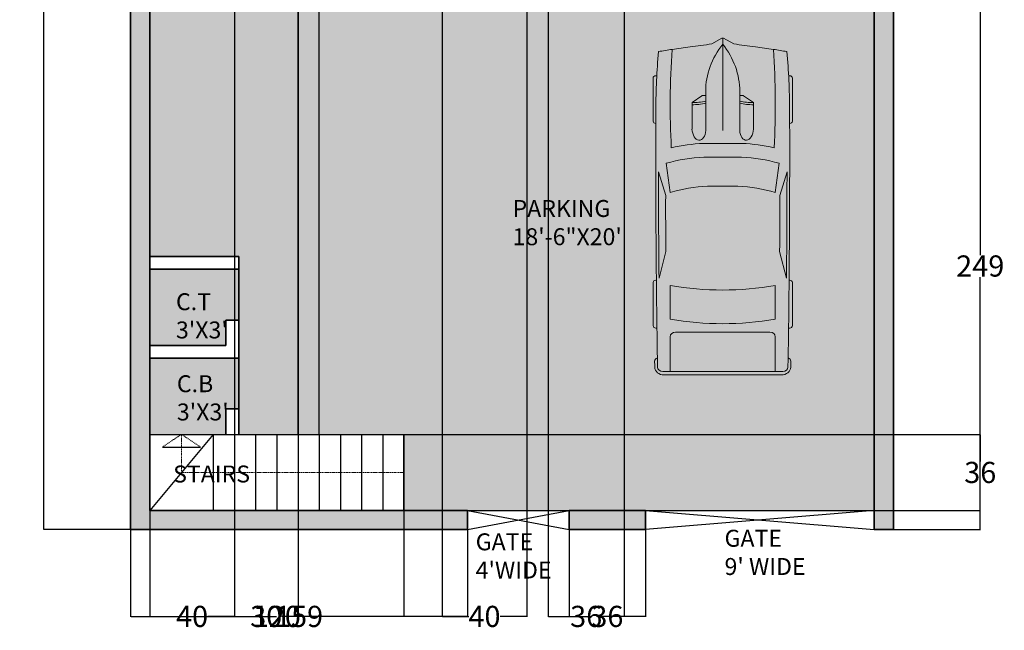
# Model space of a CAD drawing. Units: inches. Extents: x 286 to 756, y 360 to 1175.
# Tile 1 of 4: x 286 to 750, y 360 to 649. Entities that reach past the tile are written whole.
import ezdxf

# ---------------------------------------------------------------- set-up
doc = ezdxf.new("R2010")
doc.units = ezdxf.units.IN
doc.header["$MEASUREMENT"] = 0
doc.linetypes.add('DASHED', pattern=[0.75, 0.5, -0.25])
for name, color, linetype, lineweight in [('A-ANNO-DIMS', 2, 'Continuous', 18), ('A-ANNO-STRS', 7, 'DASHED', 13), ('A-ANNO-TEXT', 7, 'Continuous', 18), ('A-AREA-IDEN', 7, 'Continuous', 18), ('A-FLOR-STRS', 7, 'Continuous', 25), ('A-SITE-GATE', 4, 'Continuous', 25), ('A-WALL', 7, 'Continuous', 35), ('CAR', 8, 'Continuous', 13)]:
    doc.layers.add(name, color=color, linetype=linetype, lineweight=lineweight)
doc.layers.add('A-FLOR-PATT', color=9, linetype='Continuous', lineweight=13, true_color=0xc7c8ca)
doc.layers.add('A-WALL-PATT', color=18, linetype='Continuous', lineweight=13, true_color=0x000000)
doc.styles.get("Standard").update_dxf_attribs({"font": 'arial.ttf'})
doc.dimstyles.get("Standard").update_dxf_attribs({"dimtxt": 10, "dimasz": 0.18, "dimexe": 0.18, "dimexo": 0.0625, "dimgap": 0.09, "dimtad": 0, "dimtih": 1, "dimtoh": 1, "dimdec": 0, "dimzin": 0, "dimdsep": 46, "dimlunit": 3, "dimtxsty": 'Standard', "dimcen": 0.09, "dimadec": 0, "dimazin": 0, "dimtfac": 1, "dimtdec": 0, "dimtofl": 0, "dimtmove": 0, "dimatfit": 3, "dimfxl": 1, "dimtolj": 1, "dimtzin": 0, "dimarcsym": 0})

# ---------------------------------------------------------------- blocks, each defined once
blk = doc.blocks.new('*U4')
for p, q in [((46.55, 38.89), (22.35, 38.89)), ((136.7, 38.89), (160.9, 38.89)), ((21.1, 37.41), (21.1, 36.83)), ((47.8, 37.39), (47.8, 37.41)), ((87.99, 31.87), (74.76, 35.92)), ((134.31, 35.6), (119.29, 31.78)), ((135.45, 37.07), (135.45, 37.41)), ((162.15, 37.41), (162.15, 36.77)), ((186.47, -33.5), (186.47, 33.5)), ((70.03, 31.54), (86.41, 29.35)), ((138.42, 29.35), (157.25, 29.35)), ((186.47, 29.35), (167.01, 29.35)), ((188.4, -32.76), (188.4, 32.76)), ((164.52, 26.39), (164.52, -26.39)), ((32.27, 11.63), (36.13, 17.17)), ((36.13, 17.17), (50.94, 17.17)), ((32.12, 9.51), (32.12, 11.15)), ((3.27, 6.13), (0.1, 0.41)), ((29.77, 9.51), (51.68, 9.51)), ((58.92, -10.77), (58.92, 10.77)), ((66.55, -10.53), (66.55, 10.53)), ((82.74, 8.5), (82.74, -8.5)), ((186.47, -10.53), (186.47, 10.53)), ((0, 0), (51.68, 0)), ((0.1, -0.41), (3.27, -6.13)), ((29.77, -9.51), (51.68, -9.51)), ((32.12, -9.51), (32.12, -11.15)), ((32.27, -11.63), (36.13, -17.17)), ((36.13, -17.17), (50.94, -17.17)), ((86.41, -29.35), (70.03, -31.54)), ((87.99, -31.87), (74.76, -35.92)), ((134.31, -35.6), (119.29, -31.78)), ((157.25, -29.35), (138.42, -29.35)), ((167.01, -29.35), (186.47, -29.35)), ((21.1, -37.41), (21.1, -36.83)), ((47.8, -37.39), (47.8, -37.41)), ((135.45, -37.07), (135.45, -37.41)), ((162.15, -37.41), (162.15, -36.77)), ((46.55, -38.89), (22.35, -38.89)), ((136.7, -38.89), (160.9, -38.89))]:
    blk.add_line(p, q)
for centre, major_axis, ratio, start_param, end_param in [((22.35, 37.41), (0, -1.48), 0.842304, 3.141593, 4.712389), ((46.55, 37.41), (0, 1.48), 0.842304, -1.570796, 0), ((136.7, 37.41), (0, -1.48), 0.842304, 3.141593, 4.712389), ((160.9, 37.41), (0, 1.48), 0.842304, -1.570796, 0), ((266.03, -27.52), (0, 313.31), 0.842304, 1.367076, 1.39176), ((41.19, -490.86), (0, 528.23), 0.842304, 0.00281, 0.075598), ((64.48, -10555.62), (0, 10593.03), 0.842304, -0.013397, 0.002797), ((64.48, -10555.62), (0, -10591.55), 0.842304, 3.133765, 3.140441), ((180.63, 35.84), (0, 2.22), 0.842304, -0.013017, 1.249894), ((64.48, -10556.36), (0, 10595.31), 0.842304, -0.013397, -0.013017), ((183.98, 33.5), (0, -2.96), 0.842304, 1.570796, 3.128196), ((183.98, 32.76), (0, -5.25), 0.842304, 1.570796, 3.128196), ((259.18, -27.52), (0, -305.3), 0.842304, 4.528606, 4.561838), ((37.47, -593.96), (0, -623.33), 0.842304, 3.096046, 3.200911), ((134.4, 5.39), (0, -89.78), 0.842304, 4.449482, 4.652344), ((135.29, 5.39), (0, 81.77), 0.842304, 1.245306, 1.50788), ((149.6, 2.8), (0, -79.58), 0.842304, 4.372215, 4.640744), ((95.79, -3666.35), (0, -3698.24), 0.842304, 3.134049, 3.144098), ((17.08, 0), (0, 147.02), 0.842304, 4.511394, 4.913384), ((35.91, 0), (0, 147.02), 0.842304, 4.511394, 4.913384), ((167.01, 26.39), (0, 2.96), 0.842304, 0, 1.570796), ((-204.49, 52.4), (0, -250.96), 0.842304, 1.385369, 1.434372), ((13.04, 17.01), (0, 27.42), 0.842304, 4.435146, 4.718221), ((14.2, 17.01), (0, 27.42), 0.842304, 4.435146, 4.718221), ((50.79, 13.34), (6.34, -0.36), 0.603834, -1.395552, 1.581315), ((32.75, 11.15), (0, 0.74), 0.842304, 0.879714, 1.570796), ((29.77, -46.66), (0, 56.17), 0.842304, 0, 0.590319), ((0.62, 0), (0, -0.74), 0.842304, 4.131459, 5.293319), ((29.77, 46.66), (0, 56.17), 0.842304, 2.551274, 3.141593), ((-204.49, -52.4), (0, 250.96), 0.842304, -1.434372, -1.385369), ((13.04, -17.01), (0, -27.42), 0.842304, 1.564964, 1.848039), ((14.2, -17.01), (0, -27.42), 0.842304, 1.564964, 1.848039), ((134.4, -5.39), (0, -89.78), 0.842304, -1.510751, -1.307889), ((135.29, -5.39), (0, -81.77), 0.842304, -1.50788, -1.245306), ((149.6, -2.8), (0, -79.58), 0.842304, -1.499151, -1.230623), ((32.75, -11.15), (0, -0.74), 0.842304, 4.712389, 5.403472), ((259.18, 27.52), (0, 305.3), 0.842304, 1.721348, 1.754579), ((167.01, -26.39), (0, -2.96), 0.842304, 4.712389, 6.283185), ((266.03, 27.52), (0, 313.31), 0.842304, 1.749832, 1.774517), ((37.47, 593.96), (0, -623.33), 0.842304, -0.059319, 0.045547), ((95.79, 3666.35), (0, -3698.24), 0.842304, -0.002505, 0.007544), ((183.98, -32.76), (0, -5.25), 0.842304, 0.013397, 1.570796), ((41.19, 490.86), (0, -528.23), 0.842304, -0.075598, -0.00281), ((22.35, -37.41), (0, 1.48), 0.842304, 1.570796, 3.141593), ((64.48, 10555.62), (0, 10593.03), 0.842304, 3.138796, 3.15499), ((46.55, -37.41), (0, -1.48), 0.842304, 0, 1.570796), ((64.48, 10555.62), (0, -10591.55), 0.842304, 0.001152, 0.007828), ((136.7, -37.41), (0, -1.48), 0.842304, -1.570796, 0), ((160.9, -37.41), (0, 1.48), 0.842304, 3.141593, 4.712389), ((180.63, -35.84), (0, -2.22), 0.842304, -1.249894, 0.013017), ((64.48, 10556.36), (0, 10595.31), 0.842304, 3.15461, 3.15499), ((183.98, -33.5), (0, 2.96), 0.842304, 3.15499, 4.712389)]:
    blk.add_ellipse(centre, major_axis=major_axis, ratio=ratio, start_param=start_param, end_param=end_param)
at = {"extrusion": (0, 0, -1)}
blk.add_ellipse((50.79, -13.34), major_axis=(6.34, 0.36), ratio=0.603834, start_param=-1.395552, end_param=1.581315, dxfattribs=at)
blk = doc.blocks.new('*D22')
at = {"layer": 'A-ANNO-DIMS', "color": 0, "lineweight": -2, "transparency": 16777216}
for p, q in [((337.8, 1127.76), (296.69, 1127.76)), ((296.87, 1127.58), (296.87, 772.95)), ((296.87, 407.94), (296.87, 762.56)), ((337.8, 407.76), (296.69, 407.76))]:
    blk.add_line(p, q, dxfattribs=at)
at = {"layer": 'A-ANNO-DIMS', "color": 0, "transparency": 16777216}
for points in [[(296.84, 1127.58), (296.9, 1127.58), (296.87, 1127.76)], [(296.84, 407.94), (296.9, 407.94), (296.87, 407.76)]]:
    blk.add_solid(points, dxfattribs=at)
at = {"layer": 'Defpoints', "color": 0, "transparency": 16777216}
for p in [(296.87, 1127.76), (337.87, 1127.76), (337.87, 407.76)]:
    blk.add_point(p, dxfattribs=at)
at = {"layer": 'A-ANNO-DIMS', "color": 0, "transparency": 16777216, "insert": (296.87, 767.76), "char_height": 10, "attachment_point": 5}
blk.add_mtext('\\A1;720', dxfattribs=at)
blk = doc.blocks.new('*D23')
at = {"layer": 'A-ANNO-DIMS', "color": 0, "lineweight": -2, "transparency": 16777216}
for p, q in [((337.87, 407.69), (337.87, 366.58)), ((496.87, 407.69), (496.87, 366.58)), ((338.05, 366.76), (406.69, 366.76)), ((496.69, 366.76), (428.04, 366.76))]:
    blk.add_line(p, q, dxfattribs=at)
at = {"layer": 'A-ANNO-DIMS', "color": 0, "transparency": 16777216}
for points in [[(338.05, 366.79), (338.05, 366.73), (337.87, 366.76)], [(496.69, 366.79), (496.69, 366.73), (496.87, 366.76)]]:
    blk.add_solid(points, dxfattribs=at)
at = {"layer": 'Defpoints', "color": 0, "transparency": 16777216}
for p in [(337.87, 407.76), (496.87, 407.76), (496.87, 366.76)]:
    blk.add_point(p, dxfattribs=at)
at = {"layer": 'A-ANNO-DIMS', "color": 0, "transparency": 16777216, "insert": (417.37, 366.76), "char_height": 10, "attachment_point": 5}
blk.add_mtext('\\A1;159', dxfattribs=at)
blk = doc.blocks.new('*D24')
at = {"layer": 'A-ANNO-DIMS', "color": 0, "lineweight": -2, "transparency": 16777216}
for p, q in [((544.87, 407.69), (544.87, 366.58)), ((580.87, 407.69), (580.87, 366.58)), ((545.05, 366.76), (555.62, 366.76)), ((580.69, 366.76), (570.11, 366.76))]:
    blk.add_line(p, q, dxfattribs=at)
at = {"layer": 'A-ANNO-DIMS', "color": 0, "transparency": 16777216}
for points in [[(545.05, 366.79), (545.05, 366.73), (544.87, 366.76)], [(580.69, 366.79), (580.69, 366.73), (580.87, 366.76)]]:
    blk.add_solid(points, dxfattribs=at)
at = {"layer": 'Defpoints', "color": 0, "transparency": 16777216}
for p in [(544.87, 407.76), (580.87, 407.76), (580.87, 366.76)]:
    blk.add_point(p, dxfattribs=at)
at = {"layer": 'A-ANNO-DIMS', "color": 0, "transparency": 16777216, "insert": (562.87, 366.76), "char_height": 10, "attachment_point": 5}
blk.add_mtext('\\A1;36', dxfattribs=at)
blk = doc.blocks.new('*D25')
at = {"layer": 'A-ANNO-DIMS', "color": 0, "lineweight": -2, "transparency": 16777216}
for p, q in [((688.93, 656.76), (739.05, 656.76)), ((738.87, 656.58), (738.87, 537.45)), ((738.87, 407.94), (738.87, 527.06)), ((697.93, 407.76), (739.05, 407.76))]:
    blk.add_line(p, q, dxfattribs=at)
at = {"layer": 'A-ANNO-DIMS', "color": 0, "transparency": 16777216}
for points in [[(738.84, 656.58), (738.9, 656.58), (738.87, 656.76)], [(738.84, 407.94), (738.9, 407.94), (738.87, 407.76)]]:
    blk.add_solid(points, dxfattribs=at)
at = {"layer": 'Defpoints', "color": 0, "transparency": 16777216}
for p in [(688.87, 656.76), (738.87, 656.76), (697.87, 407.76)]:
    blk.add_point(p, dxfattribs=at)
at = {"layer": 'A-ANNO-DIMS', "color": 0, "transparency": 16777216, "insert": (738.87, 532.26), "char_height": 10, "attachment_point": 5}
blk.add_mtext('\\A1;249', dxfattribs=at)
blk = doc.blocks.new('*D31')
at = {"layer": 'A-ANNO-DIMS', "color": 0, "lineweight": -2, "transparency": 16777216}
for p, q in [((346.87, 416.69), (346.87, 366.58)), ((466.87, 416.69), (466.87, 366.58)), ((347.05, 366.76), (396.22, 366.76)), ((466.69, 366.76), (417.51, 366.76))]:
    blk.add_line(p, q, dxfattribs=at)
at = {"layer": 'A-ANNO-DIMS', "color": 0, "transparency": 16777216}
for points in [[(347.05, 366.79), (347.05, 366.73), (346.87, 366.76)], [(466.69, 366.79), (466.69, 366.73), (466.87, 366.76)]]:
    blk.add_solid(points, dxfattribs=at)
at = {"layer": 'Defpoints', "color": 0, "transparency": 16777216}
for p in [(346.87, 416.76), (466.87, 416.76), (466.87, 366.76)]:
    blk.add_point(p, dxfattribs=at)
at = {"layer": 'A-ANNO-DIMS', "color": 0, "transparency": 16777216, "insert": (406.87, 366.76), "char_height": 10, "attachment_point": 5}
blk.add_mtext('\\A1;120', dxfattribs=at)
blk = doc.blocks.new('*D32')
at = {"layer": 'A-ANNO-DIMS', "color": 0, "lineweight": -2, "transparency": 16777216}
for p, q in [((466.93, 452.76), (739.05, 452.76)), ((738.87, 452.58), (738.87, 439.95)), ((738.87, 416.94), (738.87, 429.56)), ((466.93, 416.76), (739.05, 416.76))]:
    blk.add_line(p, q, dxfattribs=at)
at = {"layer": 'A-ANNO-DIMS', "color": 0, "transparency": 16777216}
for points in [[(738.84, 452.58), (738.9, 452.58), (738.87, 452.76)], [(738.84, 416.94), (738.9, 416.94), (738.87, 416.76)]]:
    blk.add_solid(points, dxfattribs=at)
at = {"layer": 'Defpoints', "color": 0, "transparency": 16777216}
for p in [(466.87, 452.76), (738.87, 452.76), (466.87, 416.76)]:
    blk.add_point(p, dxfattribs=at)
at = {"layer": 'A-ANNO-DIMS', "color": 0, "transparency": 16777216, "insert": (738.87, 434.76), "char_height": 10, "attachment_point": 5}
blk.add_mtext('\\A1;36', dxfattribs=at)
blk = doc.blocks.new('*D33')
at = {"layer": 'A-ANNO-DIMS', "color": 0, "lineweight": -2, "transparency": 16777216}
for p, q in [((416.87, 452.82), (416.87, 1168.94)), ((417.05, 1168.76), (426.69, 1168.76)), ((426.87, 452.82), (426.87, 1168.94)), ((426.87, 1168.76), (427.05, 1168.76))]:
    blk.add_line(p, q, dxfattribs=at)
at = {"layer": 'A-ANNO-DIMS', "color": 0, "transparency": 16777216}
for points in [[(417.05, 1168.79), (417.05, 1168.73), (416.87, 1168.76)], [(426.69, 1168.79), (426.69, 1168.73), (426.87, 1168.76)]]:
    blk.add_solid(points, dxfattribs=at)
at = {"layer": 'Defpoints', "color": 0, "transparency": 16777216}
for p in [(426.87, 1168.76), (416.87, 452.76), (426.87, 452.76)]:
    blk.add_point(p, dxfattribs=at)
at = {"layer": 'A-ANNO-DIMS', "color": 0, "transparency": 16777216, "insert": (433.81, 1168.76), "char_height": 10, "attachment_point": 5}
blk.add_mtext('\\A1;10', dxfattribs=at)
blk = doc.blocks.new('*D34')
at = {"layer": 'A-ANNO-DIMS', "color": 0, "lineweight": -2, "transparency": 16777216}
for p, q in [((346.87, 1064.69), (346.87, 366.58)), ((386.87, 1064.69), (386.87, 366.58)), ((347.05, 366.76), (359.43, 366.76)), ((386.69, 366.76), (374.3, 366.76))]:
    blk.add_line(p, q, dxfattribs=at)
at = {"layer": 'A-ANNO-DIMS', "color": 0, "transparency": 16777216}
for points in [[(347.05, 366.79), (347.05, 366.73), (346.87, 366.76)], [(386.69, 366.79), (386.69, 366.73), (386.87, 366.76)]]:
    blk.add_solid(points, dxfattribs=at)
at = {"layer": 'Defpoints', "color": 0, "transparency": 16777216}
for p in [(346.87, 1064.76), (386.87, 1064.76), (386.87, 366.76)]:
    blk.add_point(p, dxfattribs=at)
at = {"layer": 'A-ANNO-DIMS', "color": 0, "transparency": 16777216, "insert": (366.87, 366.76), "char_height": 10, "attachment_point": 5}
blk.add_mtext('\\A1;40', dxfattribs=at)
blk = doc.blocks.new('*D35')
at = {"layer": 'A-ANNO-DIMS', "color": 0, "lineweight": -2, "transparency": 16777216}
for p, q in [((386.87, 1064.69), (386.87, 366.58)), ((416.87, 1064.69), (416.87, 366.58)), ((387.05, 366.76), (394.63, 366.76)), ((416.69, 366.76), (409.1, 366.76))]:
    blk.add_line(p, q, dxfattribs=at)
at = {"layer": 'A-ANNO-DIMS', "color": 0, "transparency": 16777216}
for points in [[(387.05, 366.79), (387.05, 366.73), (386.87, 366.76)], [(416.69, 366.79), (416.69, 366.73), (416.87, 366.76)]]:
    blk.add_solid(points, dxfattribs=at)
at = {"layer": 'Defpoints', "color": 0, "transparency": 16777216}
for p in [(386.87, 1064.76), (416.87, 1064.76), (416.87, 366.76)]:
    blk.add_point(p, dxfattribs=at)
at = {"layer": 'A-ANNO-DIMS', "color": 0, "transparency": 16777216, "insert": (401.87, 366.76), "char_height": 10, "attachment_point": 5}
blk.add_mtext('\\A1;30', dxfattribs=at)
blk = doc.blocks.new('*D39')
at = {"layer": 'A-ANNO-DIMS', "color": 0, "lineweight": -2, "transparency": 16777216}
for p, q in [((484.87, 920.69), (484.87, 366.58)), ((524.87, 920.69), (524.87, 366.58)), ((485.05, 366.76), (497.43, 366.76)), ((524.69, 366.76), (512.3, 366.76))]:
    blk.add_line(p, q, dxfattribs=at)
at = {"layer": 'A-ANNO-DIMS', "color": 0, "transparency": 16777216}
for points in [[(485.05, 366.79), (485.05, 366.73), (484.87, 366.76)], [(524.69, 366.79), (524.69, 366.73), (524.87, 366.76)]]:
    blk.add_solid(points, dxfattribs=at)
at = {"layer": 'Defpoints', "color": 0, "transparency": 16777216}
for p in [(484.87, 920.76), (524.87, 920.76), (524.87, 366.76)]:
    blk.add_point(p, dxfattribs=at)
at = {"layer": 'A-ANNO-DIMS', "color": 0, "transparency": 16777216, "insert": (504.87, 366.76), "char_height": 10, "attachment_point": 5}
blk.add_mtext('\\A1;40', dxfattribs=at)
blk = doc.blocks.new('*D40')
at = {"layer": 'A-ANNO-DIMS', "color": 0, "lineweight": -2, "transparency": 16777216}
for p, q in [((534.87, 920.69), (534.87, 366.58)), ((570.87, 920.69), (570.87, 366.58)), ((535.05, 366.76), (545.62, 366.76)), ((570.69, 366.76), (560.11, 366.76))]:
    blk.add_line(p, q, dxfattribs=at)
at = {"layer": 'A-ANNO-DIMS', "color": 0, "transparency": 16777216}
for points in [[(535.05, 366.79), (535.05, 366.73), (534.87, 366.76)], [(570.69, 366.79), (570.69, 366.73), (570.87, 366.76)]]:
    blk.add_solid(points, dxfattribs=at)
at = {"layer": 'Defpoints', "color": 0, "transparency": 16777216}
for p in [(534.87, 920.76), (570.87, 920.76), (570.87, 366.76)]:
    blk.add_point(p, dxfattribs=at)
at = {"layer": 'A-ANNO-DIMS', "color": 0, "transparency": 16777216, "insert": (552.87, 366.76), "char_height": 10, "attachment_point": 5}
blk.add_mtext('\\A1;36', dxfattribs=at)

msp = doc.modelspace()

# ---------------------------------------------------------------- hatches: boundary and pattern name
at = {"layer": 'A-FLOR-PATT'}
h = msp.add_hatch(color=256, dxfattribs=at)
h.dxf.hatch_style = 1
h.paths.add_polyline_path([(526.865, 1064.756), (386.892, 1064.756), (346.865, 1064.756), (346.865, 944.756), (448.865, 944.756), (448.865, 920.756), (484.865, 920.756), (484.865, 914.756), (524.865, 914.756), (524.865, 920.756), (526.865, 920.756)])
h.paths.add_polyline_path([(418.865, 1118.756), (346.865, 1118.756), (346.865, 1070.756), (386.865, 1070.756), (386.865, 1064.756), (386.892, 1064.756), (416.865, 1064.756), (416.865, 1070.756), (418.865, 1070.756)])
h.paths.add_polyline_path([(526.865, 1118.756), (424.865, 1118.756), (424.865, 1070.756), (494.865, 1070.756), (494.865, 1064.756), (524.865, 1064.756), (524.865, 1070.756), (526.865, 1070.756)])
h.paths.add_polyline_path([(610.865, 1118.756), (532.865, 1118.756), (532.865, 1070.756), (534.865, 1070.756), (534.865, 1064.756), (564.865, 1064.756), (564.865, 1070.756), (610.865, 1070.756)])
h.paths.add_polyline_path([(688.865, 1118.756), (616.865, 1118.756), (616.865, 1070.756), (618.865, 1070.756), (618.865, 1064.756), (648.865, 1064.756), (648.865, 1070.756), (688.865, 1070.756)])
h.paths.add_polyline_path([(688.865, 1064.756), (648.865, 1064.756), (618.865, 1064.756), (532.865, 1064.756), (532.865, 920.756), (534.865, 920.756), (534.865, 914.756), (570.865, 914.756), (570.865, 920.756), (586.865, 920.756), (586.865, 944.756), (688.865, 944.756)])
h.paths.add_polyline_path([(484.865, 820.756), (478.865, 820.756), (478.865, 844.756), (454.865, 844.756), (454.865, 914.756), (346.865, 914.756), (346.865, 782.756), (478.865, 782.756), (478.865, 784.756), (484.865, 784.756)])
h.paths.add_polyline_path([(688.865, 914.756), (570.865, 914.756), (534.865, 914.756), (484.865, 914.756), (484.865, 820.756), (484.865, 784.756), (484.865, 734.577), (484.865, 662.756), (486.865, 662.756), (486.865, 656.756), (534.865, 656.756), (534.865, 662.756), (688.865, 662.756)])
h.paths.add_polyline_path([(478.865, 734.756), (484.865, 734.756), (484.865, 774.756), (478.865, 774.756), (478.865, 776.756), (388.865, 776.756), (388.865, 734.756), (370.865, 734.756), (370.865, 686.756), (478.865, 686.756)])
h.paths.add_polyline_path([(688.865, 656.756), (534.865, 656.756), (486.865, 656.756), (484.865, 656.756), (346.865, 656.756), (346.865, 536.756), (388.865, 536.756), (388.865, 530.756), (388.865, 506.756), (388.865, 488.756), (388.865, 464.756), (388.865, 452.756), (466.865, 452.756), (466.865, 416.756), (496.865, 416.756), (544.865, 416.756), (580.865, 416.756), (688.865, 416.756)])
h.paths.add_polyline_path([(388.865, 530.756), (346.865, 530.756), (346.865, 494.756), (382.865, 494.756), (382.865, 506.756), (388.865, 506.756)], flags=17)
h.paths.add_polyline_path([(382.865, 464.756), (388.865, 464.756), (388.865, 488.756), (346.865, 488.756), (346.865, 452.756), (382.865, 452.756)], flags=17)
at = {"layer": 'A-WALL-PATT'}
h = msp.add_hatch(color=256, dxfattribs=at)
h.dxf.hatch_style = 1
h.paths.add_polyline_path([(496.865, 416.756), (346.865, 416.756), (346.865, 656.756), (484.865, 656.756), (486.865, 656.756), (486.865, 662.756), (484.865, 662.756), (484.865, 734.577), (478.865, 734.577), (478.865, 662.756), (346.865, 662.756), (346.865, 686.756), (337.865, 686.756), (337.865, 407.756), (496.865, 407.756)])
h.paths.add_polyline_path([(484.865, 784.756), (478.865, 784.756), (478.865, 782.756), (346.865, 782.756), (346.865, 914.756), (406.865, 914.756), (478.865, 914.756), (478.865, 820.756), (484.865, 820.756), (484.865, 920.756), (346.865, 920.756), (346.865, 968.756), (337.865, 968.756), (337.865, 710.756), (346.865, 710.756), (346.865, 734.756), (388.865, 734.756), (388.865, 776.756), (478.865, 776.756), (478.865, 774.756), (484.865, 774.756)])
h.paths.add_polyline_path([(382.865, 776.756), (382.865, 740.756), (346.865, 740.756), (346.865, 776.756)], flags=16)
h.paths.add_polyline_path([(386.865, 1070.756), (346.865, 1070.756), (346.865, 1118.756), (418.865, 1118.756), (418.865, 1106.756), (424.865, 1106.756), (424.865, 1118.756), (526.865, 1118.756), (526.865, 1070.756), (532.865, 1070.756), (532.865, 1118.756), (610.865, 1118.756), (610.865, 1106.756), (616.865, 1106.756), (616.865, 1118.756), (688.865, 1118.756), (688.865, 1016.756), (697.865, 1016.756), (697.865, 1127.756), (337.865, 1127.756), (337.865, 1016.756), (346.865, 1016.756), (346.865, 1030.663), (346.865, 1064.756), (386.865, 1064.756)])
h.paths.add_polyline_path([(494.822, 1069.262, -0.0124335), (494.859, 1070.756), (424.865, 1070.756), (424.865, 1082.756), (418.865, 1082.756), (418.865, 1070.756), (416.865, 1070.756), (416.865, 1069.252), (416.865, 1064.756), (494.822, 1064.756)], flags=17)
h.paths.add_polyline_path([(618.865, 1069.261), (618.865, 1070.756), (616.865, 1070.756), (616.865, 1082.756), (610.865, 1082.756), (610.865, 1070.756), (564.872, 1070.756, -0.0124335), (564.909, 1069.262), (564.909, 1064.756), (618.865, 1064.756)], flags=17)
h.paths.add_polyline_path([(688.865, 1070.756), (648.865, 1070.756), (648.865, 1070.756, -0.0124418), (648.902, 1069.261), (648.902, 1064.756), (688.865, 1064.756)], flags=17)
h.paths.add_polyline_path([(697.865, 968.756), (688.865, 968.756), (688.865, 920.756), (570.865, 920.756), (570.865, 914.756), (688.865, 914.756), (688.865, 873.949), (697.865, 873.949)])
h.paths.add_polyline_path([(697.865, 825.949), (688.865, 825.949), (688.865, 756.879), (697.865, 756.879)])
h.paths.add_polyline_path([(532.865, 1064.756), (526.865, 1064.756), (526.865, 920.756), (524.865, 920.756), (524.865, 914.756), (534.865, 914.756), (534.865, 920.756), (532.865, 920.756)])
h = msp.add_hatch(color=256, dxfattribs=at)
h.dxf.hatch_style = 1
h.paths.add_polyline_path([(697.865, 708.879), (688.865, 708.879), (688.865, 662.756), (534.865, 662.756), (534.865, 656.756), (688.865, 656.756), (688.865, 407.756), (697.865, 407.756)])
h.paths.add_polyline_path([(580.865, 416.756), (544.865, 416.756), (544.865, 407.756), (580.865, 407.756)], flags=17)

# ---------------------------------------------------------------- linework, layer by layer
at = {"layer": 'A-ANNO-STRS'}
for p, q in [((361.865, 452.756), (352.865, 446.756)), ((361.865, 434.756), (361.865, 452.756)), ((370.865, 446.756), (361.865, 452.756)), ((352.865, 446.756), (370.865, 446.756)), ((466.865, 434.756), (361.865, 434.756))]:
    msp.add_line(p, q, dxfattribs=at)
at = {"layer": 'A-FLOR-STRS'}
for p, q in [((346.865, 452.756), (466.865, 452.756)), ((376.865, 452.756), (346.865, 416.756)), ((376.865, 452.756), (376.865, 416.756)), ((386.865, 452.756), (386.865, 416.756)), ((396.865, 452.756), (396.865, 416.756)), ((406.865, 452.756), (406.865, 416.756)), ((416.865, 452.756), (416.865, 416.756)), ((426.865, 452.756), (426.865, 416.756)), ((436.865, 452.756), (436.865, 416.756)), ((446.865, 452.756), (446.865, 416.756)), ((456.865, 452.756), (456.865, 416.756)), ((466.865, 452.756), (466.865, 416.756)), ((466.865, 416.756), (466.865, 452.756)), ((352.865, 446.756), (370.865, 446.756))]:
    msp.add_line(p, q, dxfattribs=at)
at = {"layer": 'A-SITE-GATE'}
for p, q in [((496.865, 416.756), (544.865, 407.756)), ((496.865, 407.756), (544.865, 416.756)), ((580.865, 416.756), (688.865, 407.756)), ((688.865, 416.756), (580.865, 407.756))]:
    msp.add_line(p, q, dxfattribs=at)
at = {"layer": 'A-WALL'}
for p, q in [((337.865, 1127.756), (337.865, 407.756)), ((697.865, 407.756), (697.865, 1127.756)), ((346.865, 656.756), (346.865, 416.756)), ((688.865, 407.756), (688.865, 656.756)), ((346.865, 536.756), (388.865, 536.756)), ((388.865, 536.756), (388.865, 530.756)), ((346.865, 530.756), (388.865, 530.756)), ((388.865, 506.756), (388.865, 530.756)), ((382.865, 506.756), (382.865, 494.756)), ((382.865, 506.756), (388.865, 506.756)), ((388.865, 506.756), (388.865, 488.756)), ((346.865, 494.756), (382.865, 494.756)), ((346.865, 488.756), (388.865, 488.756)), ((388.865, 464.756), (388.865, 488.756)), ((382.865, 464.756), (382.865, 452.756)), ((382.865, 464.756), (388.865, 464.756)), ((388.865, 464.756), (388.865, 452.756)), ((346.865, 416.756), (496.865, 416.756)), ((496.865, 407.756), (496.865, 416.756)), ((544.865, 407.756), (544.865, 416.756)), ((544.865, 416.756), (580.865, 416.756)), ((580.865, 407.756), (580.865, 416.756)), ((337.865, 407.756), (496.865, 407.756)), ((544.865, 407.756), (580.865, 407.756)), ((688.865, 407.756), (697.865, 407.756))]:
    msp.add_line(p, q, dxfattribs=at)

# ---------------------------------------------------------------- block references
at = {"layer": 'CAR', "xscale": 0.8447010867429608, "yscale": 0.8447010867429608, "zscale": 0.8447010867429608, "rotation": 270}
msp.add_blockref('*U4', (617.326, 639.939), dxfattribs=at)

# ---------------------------------------------------------------- texts
at = {"layer": 'A-ANNO-TEXT', "char_height": 8, "attachment_point": 1}
for s, insert in [("GATE\\P4'WIDE", (500.724, 405.989)), ("GATE\\P9' WIDE", (618.178, 407.672))]:
    msp.add_mtext_dynamic_manual_height_columns(s, width=59.48304, gutter_width=1, heights=[0], dxfattribs=dict(at, insert=insert))
at = {"layer": 'A-AREA-IDEN', "char_height": 8, "attachment_point": 1}
for s, insert in [('PARKING\\P18\'-6"X20\'', (518.132, 563.431)), ("C.T\\P3'X3'", (359.275, 519.395)), ("C.B\\P3'X3'", (359.701, 480.663)), ('STAIRS', (357.923, 438.025))]:
    msp.add_mtext_dynamic_manual_height_columns(s, width=59.48304, gutter_width=1, heights=[0], dxfattribs=dict(at, insert=insert))

# ---------------------------------------------------------------- dimensions: what is measured, and where the dimension line sits
at = {"layer": 'A-ANNO-DIMS'}
for base, p1, p2, picture, middle in [((426.865, 1168.756), (416.865, 452.756), (426.865, 452.756), '*D33', (433.81, 1168.756)), ((386.865, 366.756), (346.865, 1064.756), (386.865, 1064.756), '*D34', (366.865, 366.756)), ((416.865, 366.756), (386.865, 1064.756), (416.865, 1064.756), '*D35', (401.865, 366.756)), ((524.865, 366.756), (484.865, 920.756), (524.865, 920.756), '*D39', (504.865, 366.756)), ((570.865, 366.756), (534.865, 920.756), (570.865, 920.756), '*D40', (552.865, 366.756)), ((466.865, 366.756), (346.865, 416.756), (466.865, 416.756), '*D31', (406.865, 366.756)), ((496.865, 366.756), (337.865, 407.756), (496.865, 407.756), '*D23', (417.365, 366.756)), ((580.865, 366.756), (544.865, 407.756), (580.865, 407.756), '*D24', (562.865, 366.756))]:
    dim = msp.add_linear_dim(base=base, p1=p1, p2=p2, dimstyle='Standard', override={"dimdec": 0, "dimlfac": 1, "dimrnd": 0, "dimzin": 0, "dimdsep": 46, "dimlunit": 2}, dxfattribs=at)
    dim.commit()
    dim.dimension.update_dxf_attribs({"geometry": picture, "text_midpoint": middle})
for base, p1, p2, picture, middle in [((296.865, 1127.756), (337.865, 407.756), (337.865, 1127.756), '*D22', (296.865, 767.756)), ((738.865, 656.756), (697.865, 407.756), (688.865, 656.756), '*D25', (738.865, 532.256)), ((738.865, 452.756), (466.865, 416.756), (466.865, 452.756), '*D32', (738.865, 434.756))]:
    dim = msp.add_linear_dim(base=base, p1=p1, p2=p2, angle=90, dimstyle='Standard', override={"dimdec": 0, "dimlfac": 1, "dimrnd": 0, "dimzin": 0, "dimdsep": 46, "dimlunit": 2}, dxfattribs=at)
    dim.commit()
    dim.dimension.update_dxf_attribs({"geometry": picture, "text_midpoint": middle})

doc.saveas('drawing.dxf')
